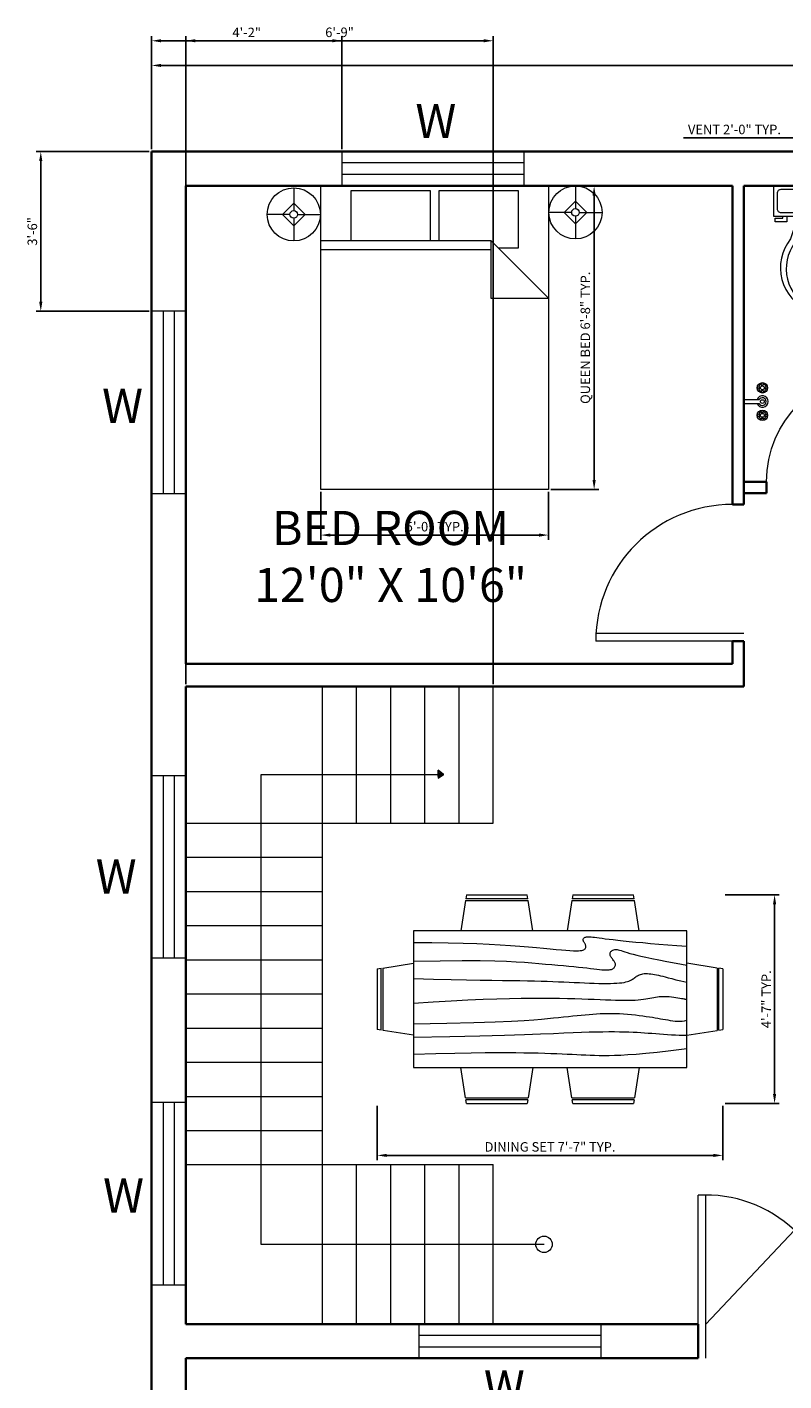
# Model space of a CAD drawing. Units: inches. Extents: x 1642 to 5612, y 1595 to 4064.
# Tile 2 of 6: x 1642 to 1842, y 1811 to 2168. Entities that reach past the tile are written whole.
import ezdxf

# ---------------------------------------------------------------- set-up
doc = ezdxf.new("R2010")
doc.units = ezdxf.units.IN
for name, color, linetype, lineweight in [('A-ANNO-DIMS', 2, 'Continuous', 18), ('A-ANNO-SYMB', 2, 'Continuous', 13), ('A-ANNO-TEXT', 7, 'Continuous', 18), ('A-AREA-IDEN', 7, 'Continuous', 25), ('A-DOOR', 3, 'Continuous', 18), ('A-FLOR-FIXT', 9, 'Continuous', 18), ('A-FLOR-STRS', 7, 'Continuous', 18), ('A-FURN', 8, 'Continuous', 13), ('A-GLAZ', 4, 'Continuous', 18), ('A-WALL', 7, 'Continuous', 35)]:
    doc.layers.add(name, color=color, linetype=linetype, lineweight=lineweight)
doc.styles.get("Standard").update_dxf_attribs({"font": 'arial.ttf'})
doc.dimstyles.new('ISO-25', dxfattribs={"dimtxt": 2.5, "dimasz": 2.5, "dimexe": 1.25, "dimexo": 0.625, "dimtad": 1, "dimdec": 0, "dimlunit": 3, "dimtxsty": 'Standard', "dimcen": 2.5, "dimadec": 0, "dimazin": 0, "dimtfac": 1, "dimtdec": 0, "dimtmove": 0, "dimatfit": 3, "dimfxl": 1, "dimarcsym": 0})

# ---------------------------------------------------------------- blocks, each defined once
blk = doc.blocks.new('Toilet - top')
for p, q in [((9.5, -6), (9.5, -2)), ((-10, -8.5), (-8, -8.5)), ((-10, -9.5), (-10, -8.5)), ((-7, -9.5), (-10, -9.5)), ((-8, -8.5), (-8, -8)), ((-7, -8), (-7, -9.5)), ((-4, -8), (-6, -14)), ((4, -8), (6, -14)), ((4, -14), (-4, -14))]:
    blk.add_line(p, q)
blk.add_lwpolyline([(10.5, -8), (10.5, 0), (-10.5, 0), (-10.5, -8)], close=True)
for points in [[(-9.5, -2), (-9.5, -6)], [(8.5, -1), (-8.5, -1)], [(-8.5, -7), (8.5, -7)]]:
    blk.add_lwpolyline(points)
for centre, radius, start, end in [((-8.62, -1.88), 0.884, 81.8699, 188.1301), ((8.62, -1.88), 0.884, 351.8699, 98.1301), ((-8.62, -6.12), 0.884, 171.8699, 278.1301), ((8.62, -6.12), 0.884, 261.8699, 8.1301), ((3.52, -21.58), 12.17, 141.4691, 247.9714), ((4.2, -21.82), 11.33, 136.3677, 238.9468), ((-3.52, -21.58), 12.17, 292.0284, 38.5307), ((-4.2, -21.82), 11.33, 301.053, 43.6321), ((0, -27.88), 4, 245.7318, 294.2682), ((0, -29), 4, 254.8605, 285.1395)]:
    blk.add_arc(centre, radius, start, end)
blk = doc.blocks.new('Faucet - Bathroom top')
for p, q in [((-4.107, 0.125), (-4.375, 0.125)), ((-3.75, 0.4788), (-3.75, 0.75)), ((-3.5, 0.482), (-3.5, 0.75)), ((-3.1461, 0.125), (-2.875, 0.125)), ((3.143, 0.125), (2.875, 0.125)), ((3.5, 0.4788), (3.5, 0.75)), ((3.75, 0.482), (3.75, 0.75)), ((4.1039, 0.125), (4.375, 0.125)), ((-4.1039, -0.125), (-4.375, -0.125)), ((-3.75, -0.4821), (-3.75, -0.75)), ((-3.5, -0.4789), (-3.5, -0.75)), ((-3.143, -0.125), (-2.875, -0.125)), ((-0.5, -0.8639), (-0.5, -4.5)), ((0.5, -4.5), (0.5, -0.8631)), ((3.1461, -0.125), (2.875, -0.125)), ((3.5, -0.4821), (3.5, -0.75)), ((3.75, -0.4789), (3.75, -0.75)), ((4.107, -0.125), (4.375, -0.125))]:
    blk.add_line(p, q)
for centre, radius in [((-3.625, 0), 1.375), ((-4.625, 0), 0.2795), ((-3.625, 0), 0.5), ((-3.625, 1), 0.2795), ((-2.625, 0), 0.2795), ((0, 0), 0.5), ((3.625, 0), 1.375), ((2.625, 0), 0.2795), ((3.625, 0), 0.5), ((3.625, 1), 0.2795), ((4.625, 0), 0.2795), ((-3.625, -1), 0.2795), ((3.625, -1), 0.2795)]:
    blk.add_circle(centre, radius)
for centre, radius, start, end in [((-3.625, 0), 1, 105.2407, 164.2093), ((-3.625, 0), 1, 16.44125, 74.07887), ((0, 0), 1.5, 289.6514, 250.3603), ((0, 0), 1, 300.3431, 239.7554), ((3.625, 0), 1, 106.12, 164.0884), ((3.625, 0), 1, 16.23422, 73.90469), ((-3.625, 0), 1, 196.2342, 253.9047), ((-3.625, 0), 1, 286.12, 344.0884), ((3.625, 0), 1, 196.4413, 254.0789), ((3.625, 0), 1, 285.2407, 344.2093), ((0, -4.5), 0.5, 180, 0)]:
    blk.add_arc(centre, radius, start, end)
blk = doc.blocks.new('Bed - Queen')
for p, q in [((0, -80.00003), (0, 0)), ((0, 0), (59.99999, 0)), ((59.99999, 0), (59.99999, -80.00003)), ((7.99999, -1.2), (28.79998, -1.2)), ((7.99999, -14.4), (7.99999, -1.2)), ((28.79998, -1.2), (28.79998, -14.4)), ((31.19999, -1.2), (51.99999, -1.2)), ((31.19999, -14.4), (31.19999, -1.2)), ((51.99999, -1.2), (51.99999, -16.4)), ((0, -14.4), (44.8, -14.4)), ((44.8, -16.8), (0, -16.8)), ((59.99999, -29.6), (44.8, -14.4)), ((44.8, -14.4), (44.8, -29.6)), ((51.99999, -16.4), (46.79936, -16.4)), ((44.8, -29.6), (59.99999, -29.6)), ((59.99999, -80.00003), (0, -80.00003))]:
    blk.add_line(p, q)
blk = doc.blocks.new('Lamp - Table')
for p, q in [((0, 7), (0, 1)), ((-1, 0), (-7, 0)), ((0, 3), (-3, 0)), ((-3, 0), (0, -3)), ((3, 0), (0, 3)), ((0, -3), (3, 0)), ((1, 0), (7, 0)), ((0, -1), (0, -7))]:
    blk.add_line(p, q)
for radius in [7, 1]:
    blk.add_circle((0, 0), radius)
blk = doc.blocks.new('Dining Set - 36 x 72 in.')
for p, q in [((-22.2343, 26.00059), (-23.4847, 17.99762)), ((-22.2304, 26), (-5.7608, 26)), ((-22, 27.5), (-22.1562, 26.50042)), ((-5.8416, 26.5), (-22.1534, 26.5)), ((-22, 27.5), (-6, 27.5)), ((-5.8437, 26.49966), (-6, 27.5)), ((-4.5152, 17.99762), (-5.7655, 25.99926)), ((5.7657, 26.00059), (4.5153, 17.99762)), ((5.7696, 26), (22.2392, 26)), ((6, 27.5), (5.8438, 26.50042)), ((22.1584, 26.5), (5.8466, 26.5)), ((6, 27.5), (22, 27.5)), ((22.1563, 26.49966), (22, 27.5)), ((23.4848, 17.99762), (22.2345, 25.99926)), ((36, 18), (-36, 18)), ((-36, 18), (-36, -18)), ((36, -18), (36, 18)), ((-45.5, 8), (-44.5004, 8.15617)), ((-45.5, 8), (-45.5, -8)), ((-44.5, -8.15843), (-44.5, 8.15338)), ((-44.0006, 8.23428), (-35.9976, 9.48474)), ((-44, 8.23041), (-44, -8.23915)), ((44.0006, 8.23428), (35.9976, 9.48474)), ((44, 8.23041), (44, -8.23915)), ((44.5, -8.15843), (44.5, 8.15338)), ((45.5, 8), (44.5005, 8.15617)), ((45.5, 8), (45.5, -8)), ((-44.4997, -8.15631), (-45.5, -8)), ((-35.9976, -9.48476), (-43.9993, -8.2345)), ((35.9976, -9.48476), (43.9993, -8.2345)), ((44.4997, -8.15631), (45.5, -8)), ((-36, -18), (36, -18)), ((-22.2343, -26.0006), (-23.4847, -17.99762)), ((-4.5152, -17.99762), (-5.7655, -25.99928)), ((5.7657, -26.0006), (4.5153, -17.99762)), ((23.4848, -17.99762), (22.2345, -25.99928)), ((-22.2304, -26), (-5.7608, -26)), ((-22, -27.5), (-22.1562, -26.50044)), ((-5.8416, -26.5), (-22.1534, -26.5)), ((-22, -27.5), (-6, -27.5)), ((-5.8437, -26.49967), (-6, -27.5)), ((5.7696, -26), (22.2392, -26)), ((6, -27.5), (5.8438, -26.50044)), ((22.1584, -26.5), (5.8466, -26.5)), ((6, -27.5), (22, -27.5)), ((22.1563, -26.49967), (22, -27.5))]:
    blk.add_line(p, q)
for points in [[(-36, 15), (-31.1772, 14.97754), (-26.8079, 14.91406), (-22.8538, 14.81543), (-19.276, 14.6875), (-16.0362, 14.53613), (-13.0957, 14.36718), (-10.4159, 14.18652), (-7.9583, 14), (-5.6904, 13.81315), (-3.6035, 13.63021), (-1.6954, 13.45508), (0.0365, 13.29166), (1.5945, 13.14388), (2.9811, 13.01562), (4.1988, 12.9108), (5.25, 12.83333), (6.1393, 12.78613), (6.8802, 12.76823), (7.4883, 12.77767), (7.9792, 12.8125), (8.3685, 12.87077), (8.6719, 12.95052), (8.9049, 13.0498), (9.0833, 13.16666), (9.2205, 13.29899), (9.3216, 13.44401), (9.3895, 13.59879), (9.4271, 13.76041), (9.4373, 13.92594), (9.4232, 14.09245), (9.3875, 14.257), (9.3333, 14.41666), (9.2638, 14.56917), (9.1836, 14.71484), (9.0975, 14.85465), (9.0104, 14.98958), (8.9272, 15.1206), (8.8529, 15.2487), (8.7922, 15.37483), (8.75, 15.5), (8.7305, 15.62467), (8.7344, 15.74739), (8.7617, 15.86621), (8.8125, 15.97916), (8.8867, 16.08431), (8.9844, 16.17968), (9.1055, 16.26334), (9.25, 16.33333), (9.4189, 16.38802), (9.6172, 16.42708), (9.8506, 16.45052), (10.125, 16.45833), (10.4463, 16.45052), (10.8203, 16.42708), (11.2529, 16.38802), (11.75, 16.33333), (12.3184, 16.26318), (12.9694, 16.17838), (13.7151, 16.07991), (14.5677, 15.96875), (15.5395, 15.84586), (16.6426, 15.71224), (17.8893, 15.56884), (19.2917, 15.41666), (20.859, 15.25667), (22.5879, 15.08984), (24.4721, 14.91715), (26.5052, 14.73958), (28.6809, 14.5581), (30.9929, 14.3737), (33.4347, 14.18733), (36, 14)], [(-36, 10), (-28.9766, 10.14274), (-23.1725, 10.20442), (-18.4241, 10.19775), (-14.5677, 10.13541), (-11.4399, 10.03011), (-8.877, 9.89453), (-6.7154, 9.74137), (-4.7917, 9.58333), (-2.9698, 9.43082), (-1.2246, 9.28515), (0.4415, 9.14534), (2.026, 9.01041), (3.5266, 8.87939), (4.9408, 8.7513), (6.266, 8.62516), (7.5, 8.5), (8.6411, 8.37549), (9.6914, 8.2539), (10.6538, 8.13818), (11.5312, 8.03125), (12.3267, 7.93603), (13.043, 7.85547), (13.6831, 7.79248), (14.25, 7.75), (14.7471, 7.7303), (15.1797, 7.73307), (15.5537, 7.75732), (15.875, 7.80208), (16.1494, 7.86637), (16.3828, 7.94922), (16.5811, 8.04964), (16.75, 8.16666), (16.8944, 8.29915), (17.0143, 8.44531), (17.1089, 8.60319), (17.1771, 8.77083), (17.218, 8.94629), (17.2305, 9.1276), (17.2137, 9.31282), (17.1667, 9.5), (17.0895, 9.6875), (16.987, 9.875), (16.8649, 10.0625), (16.7292, 10.25), (16.5856, 10.4375), (16.4401, 10.625), (16.2985, 10.8125), (16.1667, 11), (16.05, 11.18733), (15.9518, 11.3737), (15.8752, 11.5581), (15.8229, 11.73958), (15.798, 11.91715), (15.8034, 12.08984), (15.842, 12.25667), (15.9167, 12.41666), (16.0295, 12.56836), (16.1784, 12.70833), (16.3605, 12.83268), (16.5729, 12.9375), (16.8127, 13.01888), (17.0768, 13.07291), (17.3625, 13.0957), (17.6667, 13.08333), (17.9894, 13.03312), (18.3418, 12.94726), (18.7382, 12.82918), (19.1927, 12.68229), (19.7195, 12.51001), (20.3327, 12.31575), (21.0465, 12.10294), (21.875, 11.875), (22.8357, 11.63354), (23.959, 11.37304), (25.2786, 11.08618), (26.8282, 10.76562), (28.6414, 10.40405), (30.752, 9.99414), (33.1936, 9.52856), (36, 9)], [(-36, 5.5), (-30.7157, 5.3348), (-26.069, 5.20963), (-21.9946, 5.11767), (-18.4271, 5.05208), (-15.3009, 5.00602), (-12.5508, 4.97265), (-10.1112, 4.94515), (-7.9167, 4.91666), (-5.909, 4.88167), (-4.0586, 4.83984), (-2.3429, 4.79215), (-0.7396, 4.73958), (0.7739, 4.6831), (2.22, 4.6237), (3.6213, 4.56233), (5, 4.5), (6.373, 4.43782), (7.7344, 4.3776), (9.0723, 4.32129), (10.375, 4.27083), (11.6309, 4.22819), (12.8281, 4.19531), (13.9551, 4.17415), (15, 4.16666), (15.954, 4.17448), (16.819, 4.19791), (17.6001, 4.23698), (18.3021, 4.29166), (18.9299, 4.36198), (19.4883, 4.44791), (19.9823, 4.54948), (20.4167, 4.66666), (20.7969, 4.79899), (21.1302, 4.94401), (21.4245, 5.09879), (21.6875, 5.26041), (21.9271, 5.42594), (22.1511, 5.59245), (22.3672, 5.757), (22.5834, 5.91666), (22.8065, 6.06868), (23.0404, 6.21093), (23.2879, 6.34147), (23.5521, 6.45833), (23.8358, 6.55957), (24.142, 6.64323), (24.4735, 6.70735), (24.8334, 6.75), (25.2235, 6.76969), (25.642, 6.76692), (26.0858, 6.74267), (26.5521, 6.69791), (27.0379, 6.63362), (27.5404, 6.55078), (28.0565, 6.45036), (28.5834, 6.33333), (29.1242, 6.19987), (29.7071, 6.04687), (30.3661, 5.87044), (31.1354, 5.66666), (32.0493, 5.43164), (33.142, 5.16146), (34.4475, 4.85221), (36, 4.5)], [(-36, -1), (-30.7915, -0.6591), (-26.0195, -0.38216), (-21.6519, -0.16284), (-17.6563, 0.00521), (-14.0005, 0.12833), (-10.6523, 0.21289), (-7.5796, 0.26522), (-4.75, 0.29166), (-2.134, 0.29793), (0.2878, 0.28711), (2.5317, 0.26163), (4.6146, 0.22396), (6.5529, 0.17651), (8.3633, 0.12174), (10.0623, 0.06209), (11.6667, 0), (13.1899, -0.06201), (14.6341, -0.1211), (15.9982, -0.17432), (17.2813, -0.21875), (18.4823, -0.25147), (19.6003, -0.26953), (20.6343, -0.27002), (21.5834, -0.25), (22.4481, -0.20768), (23.2357, -0.14584), (23.9549, -0.06836), (24.6146, 0.02083), (25.2235, 0.11784), (25.7904, 0.21875), (26.3241, 0.31966), (26.8334, 0.41666), (27.3265, 0.50618), (27.8099, 0.58593), (28.2894, 0.65397), (28.7709, 0.70833), (29.2601, 0.74707), (29.763, 0.76823), (30.2855, 0.76985), (30.8334, 0.75), (31.4088, 0.70784), (31.9994, 0.64713), (32.589, 0.57275), (33.1615, 0.48958), (33.7008, 0.4025), (34.1908, 0.3164), (34.6153, 0.23616), (34.9584, 0.16666), (35.2099, 0.11165), (35.3848, 0.07031), (35.504, 0.04069), (35.5886, 0.02083), (35.6594, 0.00879), (35.7377, 0.0026), (35.8442, 0.00032), (36, 0)], [(-36, -6.5), (-27.1843, -6.31267), (-20.084, -6.1263), (-14.469, -5.9419), (-10.1094, -5.76042), (-6.7752, -5.58285), (-4.2363, -5.41016), (-2.2629, -5.24333), (-0.625, -5.08334), (0.8708, -4.93099), (2.2715, -4.78646), (3.5872, -4.64974), (4.8281, -4.52084), (6.0046, -4.39974), (7.127, -4.28646), (8.2053, -4.18099), (9.25, -4.08334), (10.2705, -3.99382), (11.2734, -3.91407), (12.2647, -3.84603), (13.25, -3.79167), (14.2354, -3.75293), (15.2266, -3.73177), (16.2295, -3.73015), (17.25, -3.75), (18.2912, -3.79248), (19.3451, -3.85547), (20.4009, -3.93604), (21.4479, -4.03125), (22.4754, -4.13819), (23.4727, -4.25391), (24.4289, -4.37549), (25.3334, -4.5), (26.1785, -4.62492), (26.9694, -4.74935), (27.7145, -4.87281), (28.4219, -4.99479), (29.1, -5.11483), (29.7572, -5.23242), (30.4016, -5.34709), (31.0417, -5.45834), (31.6837, -5.56437), (32.3262, -5.65821), (32.9658, -5.73153), (33.599, -5.77604), (34.2224, -5.78345), (34.8327, -5.74545), (35.4264, -5.65373), (36, -5.5)], [(-36, -10), (-26.4022, -9.81299), (-18.4675, -9.62891), (-11.9839, -9.45069), (-6.7396, -9.28125), (-2.5226, -9.12354), (0.8789, -8.98047), (3.6769, -8.85498), (6.0833, -8.75), (8.2767, -8.66765), (10.3021, -8.60677), (12.1712, -8.56543), (13.8958, -8.54167), (15.4876, -8.53353), (16.9583, -8.53907), (18.3197, -8.55632), (19.5834, -8.58334), (20.7616, -8.61841), (21.8685, -8.66081), (22.9188, -8.71004), (23.9271, -8.76563), (24.9081, -8.82707), (25.8763, -8.89388), (26.8465, -8.96558), (27.8334, -9.04167), (28.8474, -9.12118), (29.8828, -9.20117), (30.93, -9.27824), (31.9792, -9.34896), (33.0205, -9.40991), (34.0443, -9.45768), (35.0407, -9.48885), (36, -9.5)], [(-36, -14.5), (-30.0881, -14.33513), (-25.0332, -14.21224), (-20.7312, -14.12647), (-17.0781, -14.07292), (-13.97, -14.04671), (-11.3027, -14.04297), (-8.9724, -14.05681), (-6.875, -14.08334), (-4.9224, -14.11833), (-3.0905, -14.16016), (-1.3709, -14.20785), (0.2448, -14.26042), (1.7647, -14.3169), (3.1973, -14.3763), (4.5507, -14.43767), (5.8333, -14.5), (7.0554, -14.5621), (8.235, -14.62175), (9.3922, -14.67652), (10.5469, -14.72396), (11.7192, -14.76164), (12.929, -14.78711), (14.1965, -14.79794), (15.5417, -14.79167), (16.9933, -14.76424), (18.6152, -14.70508), (20.4804, -14.60197), (22.6615, -14.44271), (25.2312, -14.21509), (28.2624, -13.9069), (31.8277, -13.50594), (36, -13)]]:
    blk.add_lwpolyline(points)
blk = doc.blocks.new('*D10')
at = {"layer": 'A-ANNO-DIMS', "color": 0, "lineweight": -2, "transparency": 16777216}
for p, q in [((1675.28, 2135.62), (1675.28, 2158.94)), ((2035.28, 2135.62), (2035.28, 2158.94)), ((1677.78, 2157.69), (2032.78, 2157.69))]:
    blk.add_line(p, q, dxfattribs=at)
at = {"layer": 'A-ANNO-DIMS', "color": 0, "transparency": 16777216}
for points in [[(1677.78, 2158.1), (1677.78, 2157.27), (1675.28, 2157.69)], [(2032.78, 2158.1), (2032.78, 2157.27), (2035.28, 2157.69)]]:
    blk.add_solid(points, dxfattribs=at)
at = {"layer": 'Defpoints', "color": 0, "transparency": 16777216}
for p in [(2035.28, 2157.69), (1675.28, 2134.99), (2035.28, 2134.99)]:
    blk.add_point(p, dxfattribs=at)
at = {"layer": 'A-ANNO-DIMS', "color": 0, "transparency": 16777216, "insert": (1855.28, 2159.59), "char_height": 2.5, "attachment_point": 5}
blk.add_mtext("30'", dxfattribs=at)
blk = doc.blocks.new('WIN-48x9')
for p, q in [((0, 48), (0, 0)), ((9, 48), (0, 48)), ((3, 48), (3, 0)), ((6, 0), (6, 48)), ((9, 0), (9, 48)), ((0, 0), (9, 0))]:
    blk.add_line(p, q)
blk = doc.blocks.new('DOOR-SWING-36')
for p, q in [((36, 2), (0, 2)), ((36, 0), (0, 0))]:
    blk.add_line(p, q)
blk.add_arc((36, 0), 36, 90, 180)
blk = doc.blocks.new('DOOR-SWING-29')
for p, q in [((0, 29), (29, 29)), ((0, 27), (29, 27))]:
    blk.add_line(p, q)
blk.add_arc((0, 29), 29, 270, 0)
blk = doc.blocks.new('*D24')
at = {"layer": 'A-ANNO-DIMS', "color": 0, "lineweight": -2, "transparency": 16777216}
for p, q in [((1780.47, 2125.91), (1793.1, 2125.91)), ((1791.85, 2048.41), (1791.85, 2123.41)), ((1780.47, 2045.91), (1793.1, 2045.91))]:
    blk.add_line(p, q, dxfattribs=at)
at = {"layer": 'A-ANNO-DIMS', "color": 0, "transparency": 16777216}
for points in [[(1791.43, 2123.41), (1792.26, 2123.41), (1791.85, 2125.91)], [(1791.43, 2048.41), (1792.26, 2048.41), (1791.85, 2045.91)]]:
    blk.add_solid(points, dxfattribs=at)
at = {"layer": 'Defpoints', "color": 0, "transparency": 16777216}
for p in [(1779.85, 2125.91), (1791.85, 2125.91), (1779.85, 2045.91)]:
    blk.add_point(p, dxfattribs=at)
at = {"layer": 'A-ANNO-DIMS', "color": 0, "transparency": 16777216, "insert": (1789.85, 2085.91), "char_height": 2.5, "attachment_point": 5, "rotation": 90}
blk.add_mtext('QUEEN BED 6\'-8" TYP.', dxfattribs=at)
blk = doc.blocks.new('*D25')
at = {"layer": 'A-ANNO-DIMS', "color": 0, "lineweight": -2, "transparency": 16777216}
for p, q in [((1719.85, 2045.29), (1719.85, 2032.66)), ((1779.85, 2045.29), (1779.85, 2032.66)), ((1722.35, 2033.91), (1777.35, 2033.91))]:
    blk.add_line(p, q, dxfattribs=at)
at = {"layer": 'A-ANNO-DIMS', "color": 0, "transparency": 16777216}
for points in [[(1722.35, 2034.33), (1722.35, 2033.5), (1719.85, 2033.91)], [(1777.35, 2034.33), (1777.35, 2033.5), (1779.85, 2033.91)]]:
    blk.add_solid(points, dxfattribs=at)
at = {"layer": 'Defpoints', "color": 0, "transparency": 16777216}
for p in [(1719.85, 2045.91), (1779.85, 2045.91), (1779.85, 2033.91)]:
    blk.add_point(p, dxfattribs=at)
at = {"layer": 'A-ANNO-DIMS', "color": 0, "transparency": 16777216, "insert": (1749.85, 2035.81), "char_height": 2.5, "attachment_point": 5}
blk.add_mtext('5\'-0" TYP.', dxfattribs=at)
blk = doc.blocks.new('*D32')
at = {"layer": 'A-ANNO-DIMS', "color": 0, "lineweight": -2, "transparency": 16777216}
for p, q in [((1844.76, 2138.58), (1815.36, 2138.58)), ((1844.76, 2135.61), (1844.76, 2139.83)), ((1866.26, 2138.58), (1847.26, 2138.58)), ((1868.76, 2135.61), (1868.76, 2139.83))]:
    blk.add_line(p, q, dxfattribs=at)
at = {"layer": 'A-ANNO-DIMS', "color": 0, "transparency": 16777216}
for points in [[(1847.26, 2139), (1847.26, 2138.17), (1844.76, 2138.58)], [(1866.26, 2139), (1866.26, 2138.17), (1868.76, 2138.58)]]:
    blk.add_solid(points, dxfattribs=at)
at = {"layer": 'Defpoints', "color": 0, "transparency": 16777216}
for p in [(1844.76, 2138.58), (1844.76, 2134.98), (1868.76, 2134.98)]:
    blk.add_point(p, dxfattribs=at)
at = {"layer": 'A-ANNO-DIMS', "color": 0, "transparency": 16777216, "insert": (1828.81, 2140.49), "char_height": 2.5, "attachment_point": 5}
blk.add_mtext('VENT 2\'-0" TYP.', dxfattribs=at)
blk = doc.blocks.new('*D46')
at = {"layer": 'A-ANNO-DIMS', "color": 0, "lineweight": -2, "transparency": 16777216}
for p, q in [((1734.73, 1883.46), (1734.73, 1869.18)), ((1825.73, 1883.46), (1825.73, 1869.18)), ((1737.23, 1870.43), (1823.23, 1870.43))]:
    blk.add_line(p, q, dxfattribs=at)
at = {"layer": 'A-ANNO-DIMS', "color": 0, "transparency": 16777216}
for points in [[(1737.23, 1870.85), (1737.23, 1870.01), (1734.73, 1870.43)], [(1823.23, 1870.85), (1823.23, 1870.01), (1825.73, 1870.43)]]:
    blk.add_solid(points, dxfattribs=at)
at = {"layer": 'Defpoints', "color": 0, "transparency": 16777216}
for p in [(1734.73, 1884.08), (1825.73, 1884.08), (1825.73, 1870.43)]:
    blk.add_point(p, dxfattribs=at)
at = {"layer": 'A-ANNO-DIMS', "color": 0, "transparency": 16777216, "insert": (1780.23, 1872.35), "char_height": 2.5, "attachment_point": 5}
blk.add_mtext('DINING SET 7\'-7" TYP.', dxfattribs=at)
blk = doc.blocks.new('*D47')
at = {"layer": 'A-ANNO-DIMS', "color": 0, "lineweight": -2, "transparency": 16777216}
for p, q in [((1826.36, 1939.08), (1840.63, 1939.08)), ((1839.38, 1886.58), (1839.38, 1936.58)), ((1826.36, 1884.08), (1840.63, 1884.08))]:
    blk.add_line(p, q, dxfattribs=at)
at = {"layer": 'A-ANNO-DIMS', "color": 0, "transparency": 16777216}
for points in [[(1838.97, 1936.58), (1839.8, 1936.58), (1839.38, 1939.08)], [(1838.97, 1886.58), (1839.8, 1886.58), (1839.38, 1884.08)]]:
    blk.add_solid(points, dxfattribs=at)
at = {"layer": 'Defpoints', "color": 0, "transparency": 16777216}
for p in [(1825.73, 1939.08), (1839.38, 1939.08), (1825.73, 1884.08)]:
    blk.add_point(p, dxfattribs=at)
at = {"layer": 'A-ANNO-DIMS', "color": 0, "transparency": 16777216, "insert": (1837.51, 1911.58), "char_height": 2.5, "attachment_point": 5, "rotation": 90}
blk.add_mtext('4\'-7" TYP.', dxfattribs=at)
blk = doc.blocks.new('*D58')
at = {"layer": 'A-ANNO-DIMS', "color": 0, "lineweight": -2, "transparency": 16777216}
for p, q in [((1684.28, 1994.62), (1684.28, 2165.44)), ((1686.78, 2164.19), (1762.78, 2164.19)), ((1765.28, 1994.62), (1765.28, 2165.44))]:
    blk.add_line(p, q, dxfattribs=at)
at = {"layer": 'A-ANNO-DIMS', "color": 0, "transparency": 16777216}
for points in [[(1686.78, 2164.61), (1686.78, 2163.78), (1684.28, 2164.19)], [(1762.78, 2164.61), (1762.78, 2163.78), (1765.28, 2164.19)]]:
    blk.add_solid(points, dxfattribs=at)
at = {"layer": 'Defpoints', "color": 0, "transparency": 16777216}
for p in [(1765.28, 2164.19), (1684.28, 1993.99), (1765.28, 1993.99)]:
    blk.add_point(p, dxfattribs=at)
at = {"layer": 'A-ANNO-DIMS', "color": 0, "transparency": 16777216, "insert": (1724.78, 2166.09), "char_height": 2.5, "attachment_point": 5}
blk.add_mtext('6\'-9"', dxfattribs=at)
blk = doc.blocks.new('*D60')
at = {"layer": 'A-ANNO-DIMS', "color": 0, "lineweight": -2, "transparency": 16777216}
for p, q in [((1675.28, 2135.62), (1675.28, 2165.44)), ((1677.78, 2164.19), (1722.89, 2164.19)), ((1725.39, 2135.62), (1725.39, 2165.44))]:
    blk.add_line(p, q, dxfattribs=at)
at = {"layer": 'A-ANNO-DIMS', "color": 0, "transparency": 16777216}
for points in [[(1677.78, 2164.61), (1677.78, 2163.78), (1675.28, 2164.19)], [(1722.89, 2164.61), (1722.89, 2163.78), (1725.39, 2164.19)]]:
    blk.add_solid(points, dxfattribs=at)
at = {"layer": 'Defpoints', "color": 0, "transparency": 16777216}
for p in [(1725.39, 2164.19), (1675.28, 2134.99), (1725.39, 2134.99)]:
    blk.add_point(p, dxfattribs=at)
at = {"layer": 'A-ANNO-DIMS', "color": 0, "transparency": 16777216, "insert": (1700.33, 2166.07), "char_height": 2.5, "attachment_point": 5}
blk.add_mtext('4\'-2"', dxfattribs=at)
blk = doc.blocks.new('*D61')
at = {"layer": 'A-ANNO-DIMS', "color": 0, "lineweight": -2, "transparency": 16777216}
for p, q in [((1674.66, 2134.99), (1644.83, 2134.99)), ((1646.08, 2095.41), (1646.08, 2132.49)), ((1674.66, 2092.91), (1644.83, 2092.91))]:
    blk.add_line(p, q, dxfattribs=at)
at = {"layer": 'A-ANNO-DIMS', "color": 0, "transparency": 16777216}
for points in [[(1645.66, 2132.49), (1646.5, 2132.49), (1646.08, 2134.99)], [(1645.66, 2095.41), (1646.5, 2095.41), (1646.08, 2092.91)]]:
    blk.add_solid(points, dxfattribs=at)
at = {"layer": 'Defpoints', "color": 0, "transparency": 16777216}
for p in [(1646.08, 2134.99), (1675.28, 2134.99), (1675.28, 2092.91)]:
    blk.add_point(p, dxfattribs=at)
at = {"layer": 'A-ANNO-DIMS', "color": 0, "transparency": 16777216, "insert": (1644.18, 2113.95), "char_height": 2.5, "attachment_point": 5, "rotation": 90}
blk.add_mtext('3\'-6"', dxfattribs=at)
blk = doc.blocks.new('*D66')
at = {"layer": 'A-ANNO-DIMS', "color": 0, "lineweight": -2, "transparency": 16777216}
for p, q in [((1862.79, 1870.03), (1846.32, 1852.55)), ((1821.28, 1825.99), (1844.6, 1850.73))]:
    blk.add_line(p, q, dxfattribs=at)
at = {"layer": 'A-ANNO-DIMS', "color": 0, "transparency": 16777216}
blk.add_solid([(1846.02, 1852.84), (1846.62, 1852.27), (1844.6, 1850.73)], dxfattribs=at)
at = {"layer": 'Defpoints', "color": 0, "transparency": 16777216}
for p in [(1844.6, 1850.73), (1821.28, 1825.99)]:
    blk.add_point(p, dxfattribs=at)
at = {"layer": 'A-ANNO-DIMS', "color": 0, "transparency": 16777216, "insert": (1857.21, 1866.88), "char_height": 2.5, "attachment_point": 5, "rotation": 46.6868}
blk.add_mtext('R2\'-10"', dxfattribs=at)

msp = doc.modelspace()

# ---------------------------------------------------------------- linework, layer by layer
at = {"layer": 'A-ANNO-SYMB'}
for p, q in [((1704.17, 1846.99), (1704.17, 1970.83)), ((1704.17, 1970.83), (1750.72, 1970.83)), ((1750.72, 1970.83), (1750.72, 1971.92)), ((1750.72, 1971.92), (1750.72, 1969.87)), ((1752.19, 1970.85), (1750.72, 1971.92)), ((1750.72, 1971.92), (1752.19, 1970.85)), ((1750.72, 1970.32), (1750.72, 1971.38)), ((1750.72, 1971.38), (1752.15, 1970.83)), ((1750.72, 1969.87), (1752.19, 1970.85)), ((1752.19, 1970.85), (1750.72, 1970.85)), ((1750.72, 1970.85), (1752.15, 1970.83)), ((1752.15, 1970.83), (1750.72, 1970.32)), ((1778.65, 1846.99), (1704.17, 1846.99))]:
    msp.add_line(p, q, dxfattribs=at)
msp.add_circle((1778.65, 1846.99), 2.16, dxfattribs=at)
at = {"layer": 'A-DOOR'}
for p, q in [((1831.28, 2007.99), (1828.28, 2007.99)), ((1819.28, 1825.99), (1819.28, 1859.93)), ((1821.28, 1825.99), (1821.28, 1859.99)), ((1821.28, 1816.99), (1821.28, 1825.99))]:
    msp.add_line(p, q, dxfattribs=at)
msp.add_arc((1821.28, 1825.99), 34, 360, 93.3723, dxfattribs=at)
at = {"layer": 'A-FLOR-STRS'}
for p, q in [((1720.28, 1825.99), (1720.28, 1993.99)), ((1729.28, 1957.99), (1729.28, 1993.99)), ((1738.28, 1957.99), (1738.28, 1993.99)), ((1747.28, 1957.99), (1747.28, 1993.99)), ((1756.28, 1957.99), (1756.28, 1993.99)), ((1765.28, 1957.99), (1765.28, 1993.99)), ((1684.28, 1957.99), (1765.28, 1957.99)), ((1684.28, 1948.99), (1720.28, 1948.99)), ((1684.28, 1939.99), (1720.28, 1939.99)), ((1684.28, 1930.99), (1720.28, 1930.99)), ((1684.28, 1921.99), (1720.28, 1921.99)), ((1684.28, 1912.99), (1720.28, 1912.99)), ((1684.28, 1903.99), (1720.28, 1903.99)), ((1684.28, 1894.99), (1720.28, 1894.99)), ((1684.28, 1885.99), (1720.28, 1885.99)), ((1684.28, 1876.99), (1720.28, 1876.99)), ((1684.28, 1867.99), (1765.28, 1867.99)), ((1729.28, 1825.99), (1729.28, 1867.99)), ((1738.28, 1825.99), (1738.28, 1867.99)), ((1747.28, 1825.99), (1747.28, 1867.99)), ((1756.28, 1825.99), (1756.28, 1867.99)), ((1765.28, 1825.99), (1765.28, 1867.99))]:
    msp.add_line(p, q, dxfattribs=at)
at = {"layer": 'A-WALL'}
for p, q in [((1675.28, 2134.99), (2035.28, 2134.99)), ((1675.28, 1594.99), (1675.28, 2134.99)), ((1684.28, 2125.99), (1828.28, 2125.99)), ((1684.28, 1999.99), (1684.28, 2125.99)), ((1828.28, 2041.99), (1828.28, 2125.99)), ((1831.28, 2125.99), (1879.28, 2125.99)), ((1831.28, 2041.99), (1831.28, 2125.99)), ((1831.28, 2047.99), (1837.28, 2047.99)), ((1831.28, 2044.99), (1837.28, 2044.99)), ((1831.28, 2044.99), (1837.28, 2044.99)), ((1837.28, 2044.99), (1837.28, 2047.99)), ((1828.28, 2041.99), (1831.28, 2041.99)), ((1828.28, 1999.99), (1828.28, 2005.99)), ((1831.28, 2005.99), (1828.28, 2005.99)), ((1831.28, 2005.99), (1828.28, 2005.99)), ((1831.28, 1999.99), (1831.28, 2005.99)), ((1831.28, 1999.99), (1831.28, 2005.99)), ((1684.28, 1999.99), (1828.28, 1999.99)), ((1831.28, 1999.99), (1831.28, 1993.99)), ((1684.28, 1993.99), (1831.28, 1993.99)), ((1684.28, 1825.99), (1684.28, 1993.99)), ((1684.28, 1825.99), (1819.28, 1825.99)), ((1819.28, 1825.99), (1819.28, 1816.99)), ((1819.28, 1816.99), (1819.28, 1825.99)), ((1684.28, 1603.99), (1684.28, 1816.99)), ((1684.28, 1816.99), (1819.28, 1816.99))]:
    msp.add_line(p, q, dxfattribs=at)

# ---------------------------------------------------------------- block references
at = {"layer": 'A-DOOR', "extrusion": (0, 0, -1), "zscale": -1, "rotation": 89.9999999999989}
msp.add_blockref('DOOR-SWING-29', (-1837.28, 2047.99), dxfattribs=at)
at = {"layer": 'A-DOOR'}
msp.add_blockref('DOOR-SWING-36', (1792.28, 2005.99), dxfattribs=at)
at = {"layer": 'A-FLOR-FIXT'}
msp.add_blockref('Toilet - top', (1849.58, 2125.95), dxfattribs=at)
at = {"layer": 'A-FLOR-FIXT', "rotation": 270}
msp.add_blockref('Faucet - Bathroom top', (1836.17, 2069.1), dxfattribs=at)
at = {"layer": 'A-FURN'}
for name, p in [('Lamp - Table', (1712.73, 2118.43)), ('Bed - Queen', (1719.85, 2125.91)), ('Lamp - Table', (1786.93, 2118.96)), ('Dining Set - 36 x 72 in.', (1780.23, 1911.58))]:
    msp.add_blockref(name, p, dxfattribs=at)
at = {"layer": 'A-GLAZ', "rotation": 269.9999999999998}
for p in [(1725.39, 2134.99), (1745.69, 1825.99)]:
    msp.add_blockref('WIN-48x9', p, dxfattribs=at)
at = {"layer": 'A-GLAZ'}
for p in [(1675.28, 2044.91), (1675.28, 1922.47), (1675.28, 1836.33)]:
    msp.add_blockref('WIN-48x9', p, dxfattribs=at)

# ---------------------------------------------------------------- texts
at = {"layer": 'A-ANNO-TEXT', "char_height": 9, "attachment_point": 1}
for insert in [(1688.76, 2147.54), (1606.23, 2072.48), (1604.55, 1948.44), (1606.49, 1864.36), (1706.8, 1813.76)]:
    msp.add_mtext_dynamic_manual_height_columns('\\pxqc;W', width=122.7897, gutter_width=12.5, heights=[0], dxfattribs=dict(at, insert=insert))
at = {"layer": 'A-AREA-IDEN', "insert": (1690.5, 2040.28), "char_height": 9, "attachment_point": 1}
msp.add_mtext_dynamic_manual_height_columns('\\pxqc;BED ROOM \\P12\'0" X 10\'6"', width=95.4247, gutter_width=12.5, heights=[0], dxfattribs=at)

# ---------------------------------------------------------------- dimensions: what is measured, and where the dimension line sits
at = {"layer": 'A-ANNO-DIMS'}
for base, p1, p2, override, picture, middle in [((1725.39, 2164.19), (1675.28, 2134.99), (1725.39, 2134.99), {"dimdec": 1, "dimlfac": 1, "dimrnd": 0, "dimzin": 1, "dimdsep": 46, "dimlunit": 4, "dimfrac": 2}, '*D60', (1700.33, 2166.07)), ((1765.28, 2164.19), (1684.28, 1993.99), (1765.28, 1993.99), {"dimdec": 1, "dimlfac": 1, "dimrnd": 0, "dimzin": 1, "dimdsep": 46, "dimlunit": 4, "dimfrac": 2}, '*D58', (1724.78, 2166.09)), ((2035.28, 2157.69), (1675.28, 2134.99), (2035.28, 2134.99), {"dimclrd": 0, "dimclre": 0, "dimclrt": 0}, '*D10', (1855.28, 2159.59))]:
    dim = msp.add_linear_dim(base=base, p1=p1, p2=p2, dimstyle='ISO-25', override=override, dxfattribs=at)
    dim.commit()
    dim.dimension.update_dxf_attribs({"geometry": picture, "text_midpoint": middle})
for base, p1, p2, angle, text, picture, middle in [((1844.76, 2138.58), (1868.76, 2134.98), (1844.76, 2134.98), 180, 'VENT <> TYP.', '*D32', (1828.81, 2140.49)), ((1791.85, 2125.91), (1779.85, 2045.91), (1779.85, 2125.91), 90, 'QUEEN BED <> TYP.', '*D24', (1789.85, 2085.91)), ((1839.38, 1939.08), (1825.73, 1884.08), (1825.73, 1939.08), 90, '<> TYP.', '*D47', (1837.51, 1911.58))]:
    dim = msp.add_linear_dim(base=base, p1=p1, p2=p2, angle=angle, text=text, dimstyle='ISO-25', override={"dimdec": 1, "dimlfac": 1, "dimrnd": 0, "dimzin": 1, "dimdsep": 46, "dimlunit": 4, "dimfrac": 2}, dxfattribs=at)
    dim.commit()
    dim.dimension.update_dxf_attribs({"geometry": picture, "text_midpoint": middle})
dim = msp.add_linear_dim(base=(1646.08, 2134.99), p1=(1675.28, 2092.91), p2=(1675.28, 2134.99), angle=90, dimstyle='ISO-25', override={"dimdec": 1, "dimlfac": 1, "dimrnd": 0, "dimzin": 1, "dimdsep": 46, "dimlunit": 4, "dimfrac": 2}, dxfattribs=at)
dim.commit()
dim.dimension.update_dxf_attribs({"geometry": '*D61', "text_midpoint": (1644.18, 2113.95)})
for base, p1, p2, text, picture, middle in [((1779.85, 2033.91), (1719.85, 2045.91), (1779.85, 2045.91), '<> TYP.', '*D25', (1749.85, 2035.81)), ((1825.73, 1870.43), (1734.73, 1884.08), (1825.73, 1884.08), 'DINING SET <> TYP.', '*D46', (1780.23, 1872.35))]:
    dim = msp.add_linear_dim(base=base, p1=p1, p2=p2, text=text, dimstyle='ISO-25', override={"dimdec": 1, "dimlfac": 1, "dimrnd": 0, "dimzin": 1, "dimdsep": 46, "dimlunit": 4, "dimfrac": 2}, dxfattribs=at)
    dim.commit()
    dim.dimension.update_dxf_attribs({"geometry": picture, "text_midpoint": middle})
dim = msp.add_radius_dim(center=(1821.28, 1825.99), mpoint=(1844.6, 1850.73), dimstyle='ISO-25', override={"dimdec": 1, "dimlfac": 1, "dimrnd": 0, "dimzin": 1, "dimdsep": 46, "dimlunit": 4, "dimfrac": 2}, dxfattribs=at)
dim.commit()
dim.dimension.update_dxf_attribs({"geometry": '*D66', "text_midpoint": (1858.6, 1865.58), "dimtype": 164})

doc.saveas('drawing.dxf')
